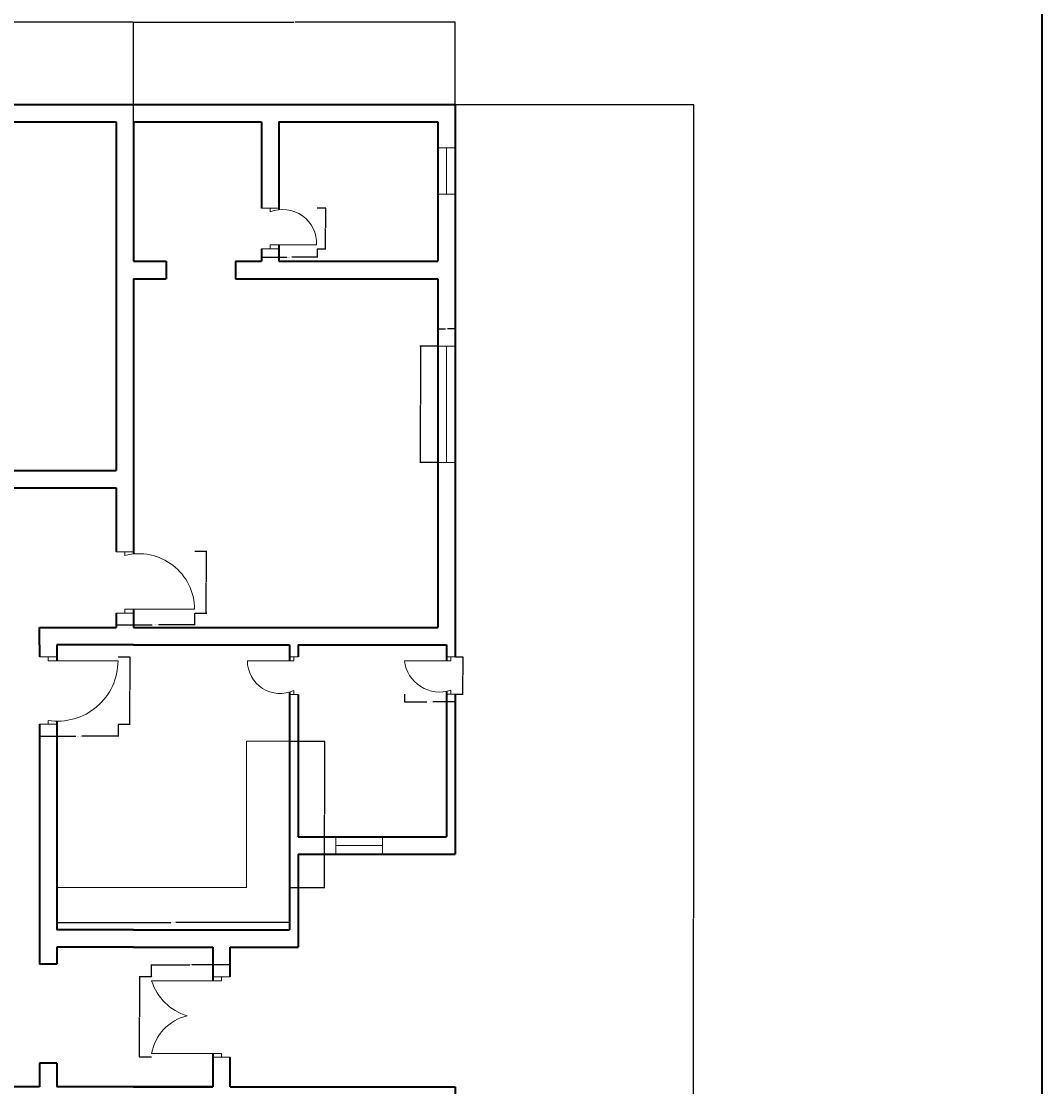
# Model space of a CAD drawing. Units: inches. Extents: x 1824 to 3509, y 619 to 2294.
# Tile 11 of 12: x 2983 to 3509, y 1115 to 1665. Entities that reach past the tile are written whole.
import ezdxf

# ---------------------------------------------------------------- set-up
doc = ezdxf.new("R2010")
doc.units = ezdxf.units.IN
for name, color, linetype, lineweight in [('A-ANNO-DIMS', 2, 'Continuous', 18), ('A-ANNO-TTLB', 7, 'Continuous', 35), ('A-DOOR', 3, 'Continuous', 18), ('A-FLOR-FIXT', 9, 'Continuous', 18), ('A-GLAZ', 4, 'Continuous', 18), ('A-WALL', 7, 'Continuous', 35)]:
    doc.layers.add(name, color=color, linetype=linetype, lineweight=lineweight)
doc.styles.get("Standard").update_dxf_attribs({"font": 'arial.ttf'})
doc.dimstyles.get("Standard").update_dxf_attribs({"dimtxt": 0.18, "dimasz": 0.18, "dimexe": 0.18, "dimexo": 0.0625, "dimgap": 0.09, "dimtad": 0, "dimtih": 1, "dimtoh": 1, "dimdec": 4, "dimzin": 0, "dimdsep": 46, "dimtxsty": 'Standard', "dimcen": 0.09, "dimadec": 0, "dimazin": 0, "dimtfac": 1, "dimtdec": 4, "dimtofl": 0, "dimtmove": 0, "dimatfit": 3, "dimfxl": 1, "dimtolj": 1, "dimtzin": 0, "dimarcsym": 0})

# ---------------------------------------------------------------- blocks, each defined once
blk = doc.blocks.new('COUNTER-L-PLAN')
for p, q in [((120, 75.53), (97.87, 75.53)), ((97.87, 75.53), (97.87, 75.53)), ((97.87, 75.53), (97.87, 0)), ((97.87, 0), (0, 0))]:
    blk.add_line(p, q)
blk = doc.blocks.new('DOOR-BATH-E-24')
for p, q in [((9, 20.96), (0, 20.96)), ((0, 20.96), (4.5, 20.96)), ((4.5, 20.96), (4.5, 20.96)), ((4.5, 20.96), (4.5, 18.96)), ((0, 0), (9, 0)), ((4.5, 0), (4.5, 2)), ((4.5, 2), (28.5, 2)), ((5.69, 0), (4.5, 0)), ((9, 0), (5.69, 0))]:
    blk.add_line(p, q)
blk.add_arc((11.01, 2.71), 17.51, 357.6736, 111.8197)
blk = doc.blocks.new('DOOR-BED-E-36')
for p, q in [((0, 31.73), (0, 31.73)), ((0, 31.73), (9, 31.73)), ((9, 31.73), (4.5, 31.73)), ((4.5, 31.73), (4.5, 29.73)), ((9, 0), (0, 0)), ((0, 0), (4.5, 0)), ((4.5, 0), (4.5, 2)), ((4.5, 2), (40.5, 2))]:
    blk.add_line(p, q)
blk.add_arc((11.82, 2), 28.68, 0, 104.7949)
blk = doc.blocks.new('DOOR-SIDE-PAIR')
for p, q in [((36, 39.48), (0, 39.48)), ((31.5, 41.48), (40.5, 41.48)), ((40.5, 41.48), (36, 41.48)), ((36, 41.48), (36, 39.48)), ((36, 2), (0, 2)), ((31.5, 0), (40.5, 0)), ((36, 0), (36, 2)), ((40.5, 0), (36, 0))]:
    blk.add_line(p, q)
for centre, radius, start, end in [((26.04, 47.53), 27.26, 197.1823, 253.5499), ((23.91, -2.24), 24.29, 103.3084, 169.936)]:
    blk.add_arc(centre, radius, start, end)
blk = doc.blocks.new('DOOR-SERVICE-EXT-24')
for p, q in [((24, 17.22), (0, 17.22)), ((21.7, 19.22), (26.2, 19.22)), ((26.2, 19.22), (24, 19.22)), ((24, 19.22), (24, 17.22)), ((21.7, 0), (26.2, 0)), ((23.95, 0), (23.95, 2)), ((26.2, 0), (23.95, 0))]:
    blk.add_line(p, q)
blk.add_arc((18.22, 19.44), 18.36, 186.9442, 288.1646)
blk = doc.blocks.new('DOOR-SERVICE-INT-24')
for p, q in [((24, 17.35), (0, 17.35)), ((21.75, 19.35), (26.25, 19.35)), ((24, 19.35), (24, 17.35)), ((21.75, 0), (26.25, 0)), ((24, 0), (24, 2)), ((26.25, 0), (24, 0))]:
    blk.add_line(p, q)
blk.add_arc((16.91, 17.35), 16.91, 180, 294.7994)
blk = doc.blocks.new('DOOR-KITCHEN-36')
for p, q in [((0, 34.79), (9, 34.79)), ((4.5, 34.79), (4.5, 32.79)), ((4.5, 32.79), (40.5, 32.79)), ((4.5, 0), (4.5, 2)), ((0, 0), (9, 0)), ((9, 0), (4.5, 0))]:
    blk.add_line(p, q)
blk.add_arc((9.34, 32.79), 31.16, 261.0709, 0)
blk = doc.blocks.new('WIN-24')
for p, q in [((0, 0), (0, 9)), ((0, 9), (0, 4.5)), ((24, 0), (24, 9)), ((0, 4.5), (24, 4.5)), ((24, 4.5), (24, 0))]:
    blk.add_line(p, q)
blk = doc.blocks.new('WIN-60')
for p, q in [((0, 9), (0, 0)), ((60, 4.5), (60, 9)), ((60, 9), (60, 0)), ((0, 0), (0, 4.5)), ((0, 4.5), (60, 4.5))]:
    blk.add_line(p, q)
blk = doc.blocks.new('*D38')
at = {"layer": 'A-ANNO-DIMS', "color": 0, "lineweight": -2, "transparency": 16777216}
for p, q in [((3197.67, 1497.24), (3188.55, 1497.24)), ((3188.73, 1497.06), (3188.73, 1467.42)), ((3188.73, 1437.42), (3188.73, 1467.06)), ((3197.67, 1437.24), (3188.55, 1437.24))]:
    blk.add_line(p, q, dxfattribs=at)
at = {"layer": 'A-ANNO-DIMS', "color": 0, "transparency": 16777216}
for points in [[(3188.7, 1497.06), (3188.76, 1497.06), (3188.73, 1497.24)], [(3188.7, 1437.42), (3188.76, 1437.42), (3188.73, 1437.24)]]:
    blk.add_solid(points, dxfattribs=at)
at = {"layer": 'Defpoints', "color": 0, "transparency": 16777216}
for p in [(3188.73, 1497.24), (3197.73, 1497.24), (3197.73, 1437.24)]:
    blk.add_point(p, dxfattribs=at)
at = {"layer": 'A-ANNO-DIMS', "color": 0, "transparency": 16777216, "insert": (3188.73, 1467.24), "char_height": 0.18, "attachment_point": 5}
blk.add_mtext('\\A1;WINDOW 60 TYP.', dxfattribs=at)
blk = doc.blocks.new('*D39')
at = {"layer": 'A-ANNO-DIMS', "color": 0, "lineweight": -2, "transparency": 16777216}
for p, q in [((3197.73, 1497.3), (3197.73, 1506.42)), ((3197.91, 1506.24), (3201.77, 1506.24)), ((3206.55, 1506.24), (3202.69, 1506.24)), ((3206.73, 1497.3), (3206.73, 1506.42))]:
    blk.add_line(p, q, dxfattribs=at)
at = {"layer": 'A-ANNO-DIMS', "color": 0, "transparency": 16777216}
for points in [[(3197.91, 1506.27), (3197.91, 1506.21), (3197.73, 1506.24)], [(3206.55, 1506.27), (3206.55, 1506.21), (3206.73, 1506.24)]]:
    blk.add_solid(points, dxfattribs=at)
at = {"layer": 'Defpoints', "color": 0, "transparency": 16777216}
for p in [(3206.73, 1506.24), (3197.73, 1497.24), (3206.73, 1497.24)]:
    blk.add_point(p, dxfattribs=at)
at = {"layer": 'A-ANNO-DIMS', "color": 0, "transparency": 16777216, "insert": (3202.23, 1506.24), "char_height": 0.18, "attachment_point": 5}
blk.add_mtext('\\A1;9 TYP.', dxfattribs=at)
blk = doc.blocks.new('*D52')
at = {"layer": 'A-ANNO-DIMS', "color": 0, "lineweight": -2, "transparency": 16777216}
for p, q in [((3001.23, 1217.79), (3001.23, 1199.67)), ((3121.23, 1217.79), (3121.23, 1199.67)), ((3001.41, 1199.85), (3059.97, 1199.85)), ((3121.05, 1199.85), (3062.48, 1199.85))]:
    blk.add_line(p, q, dxfattribs=at)
at = {"layer": 'A-ANNO-DIMS', "color": 0, "transparency": 16777216}
for points in [[(3001.41, 1199.88), (3001.41, 1199.82), (3001.23, 1199.85)], [(3121.05, 1199.88), (3121.05, 1199.82), (3121.23, 1199.85)]]:
    blk.add_solid(points, dxfattribs=at)
at = {"layer": 'Defpoints', "color": 0, "transparency": 16777216}
for p in [(3001.23, 1217.85), (3121.23, 1217.85), (3121.23, 1199.85)]:
    blk.add_point(p, dxfattribs=at)
at = {"layer": 'A-ANNO-DIMS', "color": 0, "transparency": 16777216, "insert": (3061.23, 1199.85), "char_height": 0.18, "attachment_point": 5}
blk.add_mtext('\\A1;COUNTER 120 TYP.', dxfattribs=at)
blk = doc.blocks.new('*D53')
at = {"layer": 'A-ANNO-DIMS', "color": 0, "lineweight": -2, "transparency": 16777216}
for p, q in [((3121.29, 1293.38), (3139.41, 1293.38)), ((3139.23, 1293.2), (3139.23, 1255.8)), ((3139.23, 1218.03), (3139.23, 1255.43)), ((3121.29, 1217.85), (3139.41, 1217.85))]:
    blk.add_line(p, q, dxfattribs=at)
at = {"layer": 'A-ANNO-DIMS', "color": 0, "transparency": 16777216}
for points in [[(3139.2, 1293.2), (3139.26, 1293.2), (3139.23, 1293.38)], [(3139.2, 1218.03), (3139.26, 1218.03), (3139.23, 1217.85)]]:
    blk.add_solid(points, dxfattribs=at)
at = {"layer": 'Defpoints', "color": 0, "transparency": 16777216}
for p in [(3121.23, 1293.38), (3139.23, 1293.38), (3121.23, 1217.85)]:
    blk.add_point(p, dxfattribs=at)
at = {"layer": 'A-ANNO-DIMS', "color": 0, "transparency": 16777216, "insert": (3139.23, 1255.61), "char_height": 0.18, "attachment_point": 5}
blk.add_mtext('\\A1;76 TYP.', dxfattribs=at)
blk = doc.blocks.new('*D54')
at = {"layer": 'A-ANNO-DIMS', "color": 0, "lineweight": -2, "transparency": 16777216}
for p, q in [((3106.73, 1547.53), (3106.73, 1543.1)), ((3135.47, 1547.53), (3135.47, 1543.1)), ((3106.91, 1543.28), (3119.79, 1543.28)), ((3135.29, 1543.28), (3122.41, 1543.28))]:
    blk.add_line(p, q, dxfattribs=at)
at = {"layer": 'A-ANNO-DIMS', "color": 0, "transparency": 16777216}
for points in [[(3106.91, 1543.31), (3106.91, 1543.25), (3106.73, 1543.28)], [(3135.29, 1543.31), (3135.29, 1543.25), (3135.47, 1543.28)]]:
    blk.add_solid(points, dxfattribs=at)
at = {"layer": 'Defpoints', "color": 0, "transparency": 16777216}
for p in [(3106.73, 1547.6), (3135.47, 1547.6), (3135.47, 1543.28)]:
    blk.add_point(p, dxfattribs=at)
at = {"layer": 'A-ANNO-DIMS', "color": 0, "transparency": 16777216, "insert": (3121.1, 1543.28), "char_height": 0.18, "attachment_point": 5}
blk.add_mtext('\\A1;BATH DOOR 29 TYP.', dxfattribs=at)
blk = doc.blocks.new('*D55')
at = {"layer": 'A-ANNO-DIMS', "color": 0, "lineweight": -2, "transparency": 16777216}
for p, q in [((3135.53, 1568.77), (3139.96, 1568.77)), ((3139.78, 1568.59), (3139.78, 1558.36)), ((3139.78, 1547.78), (3139.78, 1558)), ((3135.53, 1547.6), (3139.96, 1547.6))]:
    blk.add_line(p, q, dxfattribs=at)
at = {"layer": 'A-ANNO-DIMS', "color": 0, "transparency": 16777216}
for points in [[(3139.75, 1568.59), (3139.81, 1568.59), (3139.78, 1568.77)], [(3139.75, 1547.78), (3139.81, 1547.78), (3139.78, 1547.6)]]:
    blk.add_solid(points, dxfattribs=at)
at = {"layer": 'Defpoints', "color": 0, "transparency": 16777216}
for p in [(3135.47, 1568.77), (3139.78, 1568.77), (3135.47, 1547.6)]:
    blk.add_point(p, dxfattribs=at)
at = {"layer": 'A-ANNO-DIMS', "color": 0, "transparency": 16777216, "insert": (3139.78, 1558.18), "char_height": 0.18, "attachment_point": 5}
blk.add_mtext('\\A1;21 TYP.', dxfattribs=at)
blk = doc.blocks.new('*D64')
at = {"layer": 'A-ANNO-DIMS', "color": 0, "lineweight": -2, "transparency": 16777216}
for p, q in [((3031.73, 1359.41), (3031.73, 1353.22)), ((3072.23, 1359.41), (3072.23, 1353.22)), ((3031.91, 1353.4), (3050.36, 1353.4)), ((3072.05, 1353.4), (3053.6, 1353.4))]:
    blk.add_line(p, q, dxfattribs=at)
at = {"layer": 'A-ANNO-DIMS', "color": 0, "transparency": 16777216}
for points in [[(3031.91, 1353.43), (3031.91, 1353.37), (3031.73, 1353.4)], [(3072.05, 1353.43), (3072.05, 1353.37), (3072.23, 1353.4)]]:
    blk.add_solid(points, dxfattribs=at)
at = {"layer": 'Defpoints', "color": 0, "transparency": 16777216}
for p in [(3031.73, 1359.47), (3072.23, 1359.47), (3072.23, 1353.4)]:
    blk.add_point(p, dxfattribs=at)
at = {"layer": 'A-ANNO-DIMS', "color": 0, "transparency": 16777216, "insert": (3051.98, 1353.4), "char_height": 0.18, "attachment_point": 5}
blk.add_mtext('\\A1;BEDROOM DOOR 41 TYP.', dxfattribs=at)
blk = doc.blocks.new('*D65')
at = {"layer": 'A-ANNO-DIMS', "color": 0, "lineweight": -2, "transparency": 16777216}
for p, q in [((3072.29, 1391.47), (3078.48, 1391.47)), ((3078.3, 1391.29), (3078.3, 1375.65)), ((3078.3, 1359.65), (3078.3, 1375.29)), ((3072.29, 1359.47), (3078.48, 1359.47))]:
    blk.add_line(p, q, dxfattribs=at)
at = {"layer": 'A-ANNO-DIMS', "color": 0, "transparency": 16777216}
for points in [[(3078.27, 1391.29), (3078.33, 1391.29), (3078.3, 1391.47)], [(3078.27, 1359.65), (3078.33, 1359.65), (3078.3, 1359.47)]]:
    blk.add_solid(points, dxfattribs=at)
at = {"layer": 'Defpoints', "color": 0, "transparency": 16777216}
for p in [(3072.23, 1391.47), (3078.3, 1391.47), (3072.23, 1359.47)]:
    blk.add_point(p, dxfattribs=at)
at = {"layer": 'A-ANNO-DIMS', "color": 0, "transparency": 16777216, "insert": (3078.3, 1375.47), "char_height": 0.18, "attachment_point": 5}
blk.add_mtext('\\A1;32 TYP.', dxfattribs=at)
blk = doc.blocks.new('*D66')
at = {"layer": 'A-ANNO-DIMS', "color": 0, "lineweight": -2, "transparency": 16777216}
for p, q in [((3050.03, 1171.75), (3043.69, 1171.75)), ((3043.87, 1171.57), (3043.87, 1151.2)), ((3043.87, 1130.45), (3043.87, 1150.83)), ((3050.03, 1130.27), (3043.69, 1130.27))]:
    blk.add_line(p, q, dxfattribs=at)
at = {"layer": 'A-ANNO-DIMS', "color": 0, "transparency": 16777216}
for points in [[(3043.84, 1171.57), (3043.9, 1171.57), (3043.87, 1171.75)], [(3043.84, 1130.45), (3043.9, 1130.45), (3043.87, 1130.27)]]:
    blk.add_solid(points, dxfattribs=at)
at = {"layer": 'Defpoints', "color": 0, "transparency": 16777216}
for p in [(3043.87, 1171.75), (3050.09, 1171.75), (3050.09, 1130.27)]:
    blk.add_point(p, dxfattribs=at)
at = {"layer": 'A-ANNO-DIMS', "color": 0, "transparency": 16777216, "insert": (3043.87, 1151.01), "char_height": 0.18, "attachment_point": 5}
blk.add_mtext('\\A1;SIDE DOORS 41 TYP.', dxfattribs=at)
blk = doc.blocks.new('*D67')
at = {"layer": 'A-ANNO-DIMS', "color": 0, "lineweight": -2, "transparency": 16777216}
for p, q in [((3050.09, 1171.82), (3050.09, 1178.16)), ((3050.27, 1177.98), (3069.81, 1177.98)), ((3090.41, 1177.98), (3070.87, 1177.98)), ((3090.59, 1171.82), (3090.59, 1178.16))]:
    blk.add_line(p, q, dxfattribs=at)
at = {"layer": 'A-ANNO-DIMS', "color": 0, "transparency": 16777216}
for points in [[(3050.27, 1178.01), (3050.27, 1177.95), (3050.09, 1177.98)], [(3090.41, 1178.01), (3090.41, 1177.95), (3090.59, 1177.98)]]:
    blk.add_solid(points, dxfattribs=at)
at = {"layer": 'Defpoints', "color": 0, "transparency": 16777216}
for p in [(3090.59, 1177.98), (3050.09, 1171.75), (3090.59, 1171.75)]:
    blk.add_point(p, dxfattribs=at)
at = {"layer": 'A-ANNO-DIMS', "color": 0, "transparency": 16777216, "insert": (3070.34, 1177.98), "char_height": 0.18, "attachment_point": 5}
blk.add_mtext('\\A1;41 TYP.', dxfattribs=at)
blk = doc.blocks.new('*D68')
at = {"layer": 'A-ANNO-DIMS', "color": 0, "lineweight": -2, "transparency": 16777216}
for p, q in [((3180.53, 1317.64), (3180.53, 1313.6)), ((3206.73, 1317.64), (3206.73, 1313.6)), ((3180.71, 1313.78), (3192.1, 1313.78)), ((3206.55, 1313.78), (3195.16, 1313.78))]:
    blk.add_line(p, q, dxfattribs=at)
at = {"layer": 'A-ANNO-DIMS', "color": 0, "transparency": 16777216}
for points in [[(3180.71, 1313.81), (3180.71, 1313.75), (3180.53, 1313.78)], [(3206.55, 1313.81), (3206.55, 1313.75), (3206.73, 1313.78)]]:
    blk.add_solid(points, dxfattribs=at)
at = {"layer": 'Defpoints', "color": 0, "transparency": 16777216}
for p in [(3180.53, 1317.71), (3206.73, 1317.71), (3206.73, 1313.78)]:
    blk.add_point(p, dxfattribs=at)
at = {"layer": 'A-ANNO-DIMS', "color": 0, "transparency": 16777216, "insert": (3193.63, 1313.78), "char_height": 0.18, "attachment_point": 5}
blk.add_mtext('\\A1;SERVICE DOOR 26 TYP.', dxfattribs=at)
blk = doc.blocks.new('*D69')
at = {"layer": 'A-ANNO-DIMS', "color": 0, "lineweight": -2, "transparency": 16777216}
for p, q in [((3206.79, 1336.93), (3210.84, 1336.93)), ((3210.66, 1336.75), (3210.66, 1327.5)), ((3210.66, 1317.89), (3210.66, 1327.14)), ((3206.79, 1317.71), (3210.84, 1317.71))]:
    blk.add_line(p, q, dxfattribs=at)
at = {"layer": 'A-ANNO-DIMS', "color": 0, "transparency": 16777216}
for points in [[(3210.63, 1336.75), (3210.69, 1336.75), (3210.66, 1336.93)], [(3210.63, 1317.89), (3210.69, 1317.89), (3210.66, 1317.71)]]:
    blk.add_solid(points, dxfattribs=at)
at = {"layer": 'Defpoints', "color": 0, "transparency": 16777216}
for p in [(3206.73, 1336.93), (3210.66, 1336.93), (3206.73, 1317.71)]:
    blk.add_point(p, dxfattribs=at)
at = {"layer": 'A-ANNO-DIMS', "color": 0, "transparency": 16777216, "insert": (3210.66, 1327.32), "char_height": 0.18, "attachment_point": 5}
blk.add_mtext('\\A1;19 TYP.', dxfattribs=at)
blk = doc.blocks.new('*D72')
at = {"layer": 'A-ANNO-DIMS', "color": 0, "lineweight": -2, "transparency": 16777216}
for p, q in [((2992.23, 1302.08), (2992.23, 1295.89)), ((3032.73, 1302.08), (3032.73, 1295.89)), ((2992.41, 1296.07), (3010.96, 1296.07)), ((3032.55, 1296.07), (3014, 1296.07))]:
    blk.add_line(p, q, dxfattribs=at)
at = {"layer": 'A-ANNO-DIMS', "color": 0, "transparency": 16777216}
for points in [[(2992.41, 1296.1), (2992.41, 1296.04), (2992.23, 1296.07)], [(3032.55, 1296.1), (3032.55, 1296.04), (3032.73, 1296.07)]]:
    blk.add_solid(points, dxfattribs=at)
at = {"layer": 'Defpoints', "color": 0, "transparency": 16777216}
for p in [(2992.23, 1302.14), (3032.73, 1302.14), (3032.73, 1296.07)]:
    blk.add_point(p, dxfattribs=at)
at = {"layer": 'A-ANNO-DIMS', "color": 0, "transparency": 16777216, "insert": (3012.48, 1296.07), "char_height": 0.18, "attachment_point": 5}
blk.add_mtext('\\A1;KITCHEN DOOR 41 TYP.', dxfattribs=at)
blk = doc.blocks.new('*D73')
at = {"layer": 'A-ANNO-DIMS', "color": 0, "lineweight": -2, "transparency": 16777216}
for p, q in [((3032.79, 1336.93), (3038.98, 1336.93)), ((3038.8, 1336.75), (3038.8, 1319.72)), ((3038.8, 1302.32), (3038.8, 1319.35)), ((3032.79, 1302.14), (3038.98, 1302.14))]:
    blk.add_line(p, q, dxfattribs=at)
at = {"layer": 'A-ANNO-DIMS', "color": 0, "transparency": 16777216}
for points in [[(3038.77, 1336.75), (3038.83, 1336.75), (3038.8, 1336.93)], [(3038.77, 1302.32), (3038.83, 1302.32), (3038.8, 1302.14)]]:
    blk.add_solid(points, dxfattribs=at)
at = {"layer": 'Defpoints', "color": 0, "transparency": 16777216}
for p in [(3032.73, 1336.93), (3038.8, 1336.93), (3032.73, 1302.14)]:
    blk.add_point(p, dxfattribs=at)
at = {"layer": 'A-ANNO-DIMS', "color": 0, "transparency": 16777216, "insert": (3038.8, 1319.54), "char_height": 0.18, "attachment_point": 5}
blk.add_mtext('\\A1;35 TYP.', dxfattribs=at)
blk = doc.blocks.new('*D104')
at = {"layer": 'A-ANNO-DIMS', "color": 0, "lineweight": -2, "transparency": 16777216}
for p, q in [((3206.79, 1622.1), (3329.93, 1622.1)), ((3329.75, 1621.92), (3329.75, 1202.28)), ((3329.75, 782.28), (3329.75, 1201.92)), ((2875.79, 782.1), (3329.93, 782.1))]:
    blk.add_line(p, q, dxfattribs=at)
at = {"layer": 'A-ANNO-DIMS', "color": 0, "transparency": 16777216}
for points in [[(3329.72, 1621.92), (3329.78, 1621.92), (3329.75, 1622.1)], [(3329.72, 782.28), (3329.78, 782.28), (3329.75, 782.1)]]:
    blk.add_solid(points, dxfattribs=at)
at = {"layer": 'Defpoints', "color": 0, "transparency": 16777216}
for p in [(3206.73, 1622.1), (3329.75, 1622.1), (2875.73, 782.1)]:
    blk.add_point(p, dxfattribs=at)
at = {"layer": 'A-ANNO-DIMS', "color": 0, "transparency": 16777216, "insert": (3329.75, 1202.1), "char_height": 0.18, "attachment_point": 5}
blk.add_mtext('\\A1;840', dxfattribs=at)
blk = doc.blocks.new('*D116')
at = {"layer": 'A-ANNO-DIMS', "color": 0, "lineweight": -2, "transparency": 16777216}
for p, q in [((2907.5, 1622.16), (2907.5, 1664.63)), ((2907.68, 1664.45), (2973.66, 1664.45)), ((3040.55, 1664.45), (2974.57, 1664.45)), ((3040.73, 1613.16), (3040.73, 1664.63))]:
    blk.add_line(p, q, dxfattribs=at)
at = {"layer": 'A-ANNO-DIMS', "color": 0, "transparency": 16777216}
for points in [[(2907.68, 1664.48), (2907.68, 1664.42), (2907.5, 1664.45)], [(3040.55, 1664.48), (3040.55, 1664.42), (3040.73, 1664.45)]]:
    blk.add_solid(points, dxfattribs=at)
at = {"layer": 'Defpoints', "color": 0, "transparency": 16777216}
for p in [(3040.73, 1664.45), (2907.5, 1622.1), (3040.73, 1613.1)]:
    blk.add_point(p, dxfattribs=at)
at = {"layer": 'A-ANNO-DIMS', "color": 0, "transparency": 16777216, "insert": (2974.11, 1664.45), "char_height": 0.18, "attachment_point": 5}
blk.add_mtext('\\A1;133.23', dxfattribs=at)
blk = doc.blocks.new('*D117')
at = {"layer": 'A-ANNO-DIMS', "color": 0, "lineweight": -2, "transparency": 16777216}
for p, q in [((3040.73, 1613.16), (3040.73, 1664.63)), ((3040.91, 1664.45), (3123.45, 1664.45)), ((3206.55, 1664.45), (3124.01, 1664.45)), ((3206.73, 1622.16), (3206.73, 1664.63))]:
    blk.add_line(p, q, dxfattribs=at)
at = {"layer": 'A-ANNO-DIMS', "color": 0, "transparency": 16777216}
for points in [[(3040.91, 1664.48), (3040.91, 1664.42), (3040.73, 1664.45)], [(3206.55, 1664.48), (3206.55, 1664.42), (3206.73, 1664.45)]]:
    blk.add_solid(points, dxfattribs=at)
at = {"layer": 'Defpoints', "color": 0, "transparency": 16777216}
for p in [(3206.73, 1664.45), (3206.73, 1622.1), (3040.73, 1613.1)]:
    blk.add_point(p, dxfattribs=at)
at = {"layer": 'A-ANNO-DIMS', "color": 0, "transparency": 16777216, "insert": (3123.73, 1664.45), "char_height": 0.18, "attachment_point": 5}
blk.add_mtext('\\A1;166', dxfattribs=at)

msp = doc.modelspace()

# ---------------------------------------------------------------- linework, layer by layer
at = {"layer": 'A-ANNO-TTLB'}
msp.add_lwpolyline([(1824.0608, 2293.6614), (3509.3484, 2293.6614), (3509.3484, 619.4665), (1824.0608, 619.4665)], close=True, dxfattribs=at)
at = {"layer": 'A-GLAZ'}
msp.add_line((3206.7282, 1599.654), (3206.7282, 1599.654), dxfattribs=at)
at = {"layer": 'A-WALL'}
for p, q in [((2689.7282, 1622.1012), (3206.7282, 1622.1012)), ((3206.7282, 1622.1012), (3206.7282, 1336.9292)), ((2875.7282, 1613.1012), (3031.7282, 1613.1012)), ((3031.7282, 1613.1012), (3031.7282, 1433.1012)), ((3040.7282, 1613.1012), (3040.7282, 1541.1012)), ((3040.7282, 1613.1012), (3106.7282, 1613.1012)), ((3106.7282, 1613.1012), (3106.7282, 1568.5597)), ((3115.7282, 1613.1012), (3115.7282, 1567.6985)), ((3115.7282, 1613.1012), (3197.7282, 1613.1012)), ((3197.7282, 1613.1012), (3197.7282, 1541.1012)), ((3106.7282, 1547.5961), (3106.7282, 1541.1012)), ((3115.7282, 1549.5961), (3115.7282, 1541.1012)), ((3040.7282, 1541.1012), (3057.6155, 1541.1012)), ((3057.6155, 1541.1012), (3057.6155, 1532.1012)), ((3093.2754, 1541.1012), (3106.7282, 1541.1012)), ((3093.2754, 1541.1012), (3093.2754, 1532.1012)), ((3115.7282, 1541.1012), (3197.7282, 1541.1012)), ((3040.7282, 1532.1012), (3040.7282, 1390.0103)), ((3040.7282, 1532.1012), (3057.6155, 1532.1012)), ((3093.2754, 1532.1012), (3197.7282, 1532.1012)), ((3197.7282, 1532.1012), (3197.7282, 1352.1012)), ((2918.9899, 1433.1012), (3031.7282, 1433.1012)), ((2921.2717, 1424.1012), (3031.7282, 1424.1012)), ((3031.7282, 1424.1012), (3031.7282, 1391.1988)), ((3031.7282, 1359.4725), (3031.7282, 1352.1012)), ((3040.7282, 1361.4725), (3040.7282, 1352.1012)), ((2992.2282, 1343.1012), (2992.2282, 1352.1012)), ((2992.2282, 1352.1012), (3031.7282, 1352.1012)), ((3040.7282, 1352.1012), (3197.7282, 1352.1012)), ((2992.2282, 1343.1012), (2992.2282, 1336.9292)), ((3001.2282, 1343.1012), (3001.2282, 1334.9292)), ((3040.7282, 1343.1012), (3001.2282, 1343.1012)), ((3040.7282, 1343.1012), (3121.2282, 1343.1012)), ((3121.2282, 1343.1012), (3121.2282, 1334.9292)), ((3125.7282, 1343.1012), (3125.7282, 1336.9292)), ((3125.7282, 1343.1012), (3197.7282, 1343.1012)), ((3197.7282, 1343.1012), (3202.2282, 1343.1012)), ((3202.2282, 1343.1012), (3202.2282, 1334.9292)), ((3121.2282, 1318.7293), (3121.2282, 1196.1012)), ((3125.7282, 1317.5804), (3125.7282, 1244.1012)), ((3202.2282, 1319.1219), (3202.2282, 1244.1012)), ((3206.7282, 1317.7052), (3206.7282, 1235.1012)), ((3001.2282, 1303.7679), (3001.2282, 1196.1012)), ((2992.2282, 1302.1437), (2992.2282, 1178.3005)), ((3125.7282, 1244.1012), (3202.2282, 1244.1012)), ((3125.7282, 1235.1012), (3125.7282, 1187.1012)), ((3125.7282, 1235.1012), (3197.7282, 1235.1012)), ((3197.7282, 1235.1012), (3206.7282, 1235.1012)), ((3040.7282, 1196.1012), (3001.2282, 1196.1012)), ((3040.7282, 1196.1012), (3121.2282, 1196.1012)), ((3001.2282, 1187.1012), (3001.2282, 1178.3005)), ((3040.7282, 1187.1012), (3001.2282, 1187.1012)), ((3040.7282, 1187.1012), (3081.5899, 1187.1012)), ((3081.5899, 1187.1012), (3081.5899, 1169.754)), ((3090.5899, 1187.1012), (3125.7282, 1187.1012)), ((3090.5899, 1171.754), (3090.5899, 1187.1012)), ((3001.2282, 1178.3005), (2992.2282, 1178.3005)), ((2992.2282, 1127.2043), (2992.2282, 1115.1012)), ((3001.2282, 1127.2043), (2992.2282, 1127.2043)), ((3001.2282, 1127.2043), (3001.2282, 1115.1012)), ((3081.5899, 1132.2745), (3081.5899, 1115.1012)), ((3090.5899, 1115.1012), (3090.5899, 1130.2745)), ((2992.2282, 1115.1012), (2957.4861, 1115.1012)), ((3081.5899, 1115.1012), (3001.2282, 1115.1012)), ((3040.7282, 1115.1012), (3081.5899, 1115.1012)), ((3090.5899, 1115.1012), (3197.7282, 1115.1012)), ((3197.7282, 1115.1012), (3206.7282, 1115.1012)), ((3206.7282, 1115.1012), (3206.7282, 818.1012))]:
    msp.add_line(p, q, dxfattribs=at)

# ---------------------------------------------------------------- block references
at = {"layer": 'A-DOOR'}
for name, p in [('DOOR-BATH-E-24', (3106.7283, 1547.596)), ('DOOR-BED-E-36', (3031.7283, 1359.472)), ('DOOR-KITCHEN-36', (2992.2283, 1302.144)), ('DOOR-SERVICE-INT-24', (3099.4783, 1317.58)), ('DOOR-SERVICE-EXT-24', (3180.5313, 1317.705)), ('DOOR-SIDE-PAIR', (3050.0903, 1130.274))]:
    msp.add_blockref(name, p, dxfattribs=at)
at = {"layer": 'A-FLOR-FIXT'}
msp.add_blockref('COUNTER-L-PLAN', (3001.2283, 1217.851), dxfattribs=at)
at = {"layer": 'A-GLAZ', "rotation": 270}
msp.add_blockref('WIN-24', (3197.728, 1599.6544), dxfattribs=at)
at = {"layer": 'A-GLAZ', "extrusion": (0, 0, -1), "zscale": -1}
for name, p, rotation in [('WIN-60', (-3197.728, 1437.2381), 90), ('WIN-24', (-3145.2035, 1244.1013), 180)]:
    msp.add_blockref(name, p, dxfattribs=dict(at, rotation=rotation))

# ---------------------------------------------------------------- dimensions: what is measured, and where the dimension line sits
at = {"layer": 'A-ANNO-DIMS'}
for base, p1, p2, override, picture, middle in [((3040.7282, 1664.4512), (2907.4978, 1622.1012), (3040.7282, 1613.1012), {"dimdec": 2, "dimlfac": 1, "dimrnd": 0, "dimzin": 0, "dimdsep": 46, "dimlunit": 2}, '*D116', (2974.113, 1664.4512)), ((3206.7282, 1664.4512), (3040.7282, 1613.1012), (3206.7282, 1622.1012), {"dimdec": 0, "dimlfac": 1, "dimrnd": 0, "dimzin": 0, "dimdsep": 46, "dimlunit": 2}, '*D117', (3123.7282, 1664.4512))]:
    dim = msp.add_linear_dim(base=base, p1=p1, p2=p2, dimstyle='Standard', override=override, dxfattribs=at)
    dim.commit()
    dim.dimension.update_dxf_attribs({"geometry": picture, "text_midpoint": middle})
dim = msp.add_linear_dim(base=(3329.7513, 1622.1012), p1=(2875.7282, 782.1012), p2=(3206.7282, 1622.1012), angle=90, dimstyle='Standard', override={"dimdec": 0, "dimlfac": 1, "dimrnd": 0, "dimzin": 0, "dimdsep": 46, "dimlunit": 2}, dxfattribs=at)
dim.commit()
dim.dimension.update_dxf_attribs({"geometry": '*D104', "text_midpoint": (3329.7513, 1202.1012)})
for base, p1, p2, text, picture, middle in [((3139.7803, 1568.7662), (3135.4692, 1547.5961), (3135.4692, 1568.7662), '<> TYP.', '*D55', (3139.7803, 1558.1811)), ((3188.7282, 1497.2385), (3197.7282, 1437.2385), (3197.7282, 1497.2385), 'WINDOW <> TYP.', '*D38', (3188.7282, 1467.2385)), ((3078.3032, 1391.4708), (3072.2282, 1359.4725), (3072.2282, 1391.4708), '<> TYP.', '*D65', (3078.3032, 1375.4716)), ((3038.8032, 1336.9292), (3032.7282, 1302.1437), (3032.7282, 1336.9292), '<> TYP.', '*D73', (3038.8032, 1319.5365)), ((3210.6578, 1336.9292), (3206.7282, 1317.7052), (3206.7282, 1336.9292), '<> TYP.', '*D69', (3210.6578, 1327.3172)), ((3139.2282, 1293.3772), (3121.2282, 1217.8511), (3121.2282, 1293.3772), '<> TYP.', '*D53', (3139.2282, 1255.6142)), ((3043.868, 1171.754), (3050.0899, 1130.2745), (3050.0899, 1171.754), 'SIDE DOORS <> TYP.', '*D66', (3043.868, 1151.0142))]:
    dim = msp.add_linear_dim(base=base, p1=p1, p2=p2, angle=90, text=text, dimstyle='Standard', override={"dimdec": 0, "dimlfac": 1, "dimrnd": 0, "dimzin": 0, "dimdsep": 46, "dimlunit": 2}, dxfattribs=at)
    dim.commit()
    dim.dimension.update_dxf_attribs({"geometry": picture, "text_midpoint": middle})
for base, p1, p2, text, picture, middle in [((3135.4692, 1543.2849), (3106.7282, 1547.5961), (3135.4692, 1547.5961), 'BATH DOOR <> TYP.', '*D54', (3121.0987, 1543.2849)), ((3206.7282, 1506.2385), (3197.7282, 1497.2385), (3206.7282, 1497.2385), '<> TYP.', '*D39', (3202.2282, 1506.2385)), ((3072.2282102324, 1353.3974807302), (3031.7282102324, 1359.4724807302), (3072.2282102324, 1359.4724807302), 'BEDROOM DOOR <> TYP.', '*D64', (3051.9782102324, 1353.3974807302)), ((3206.7282, 1313.7757), (3180.5313, 1317.7052), (3206.7282, 1317.7052), 'SERVICE DOOR <> TYP.', '*D68', (3193.6297, 1313.7757)), ((3032.7282102324, 1296.06874232), (2992.2282102324, 1302.14374232), (3032.7282102324, 1302.14374232), 'KITCHEN DOOR <> TYP.', '*D72', (3012.4782102324, 1296.06874232)), ((3121.2282, 1199.8511), (3001.2282, 1217.8511), (3121.2282, 1217.8511), 'COUNTER <> TYP.', '*D52', (3061.2282, 1199.8511)), ((3090.5899100694, 1177.9759324114), (3050.0899100694, 1171.7540042555), (3090.5899100694, 1171.7540042555), '<> TYP.', '*D67', (3070.3399100694, 1177.9759324114))]:
    dim = msp.add_linear_dim(base=base, p1=p1, p2=p2, text=text, dimstyle='Standard', override={"dimdec": 0, "dimlfac": 1, "dimrnd": 0, "dimzin": 0, "dimdsep": 46, "dimlunit": 2}, dxfattribs=at)
    dim.commit()
    dim.dimension.update_dxf_attribs({"geometry": picture, "text_midpoint": middle})

doc.saveas('drawing.dxf')
